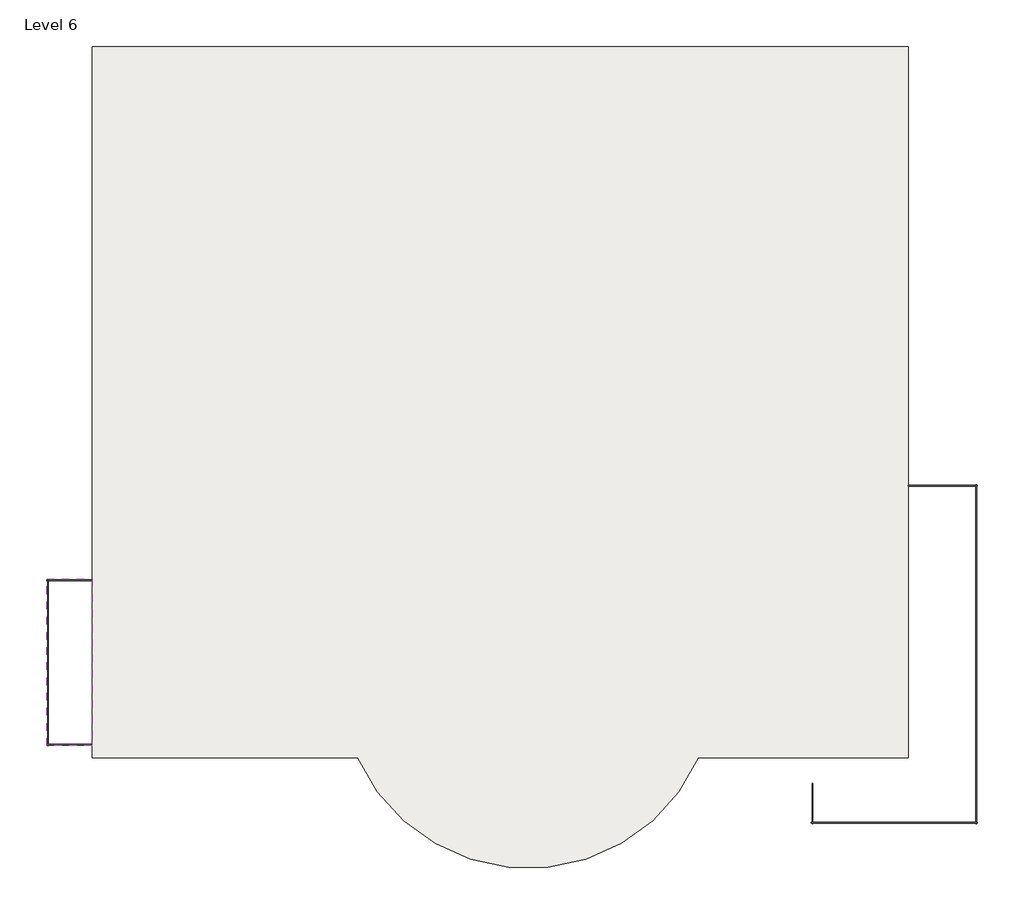
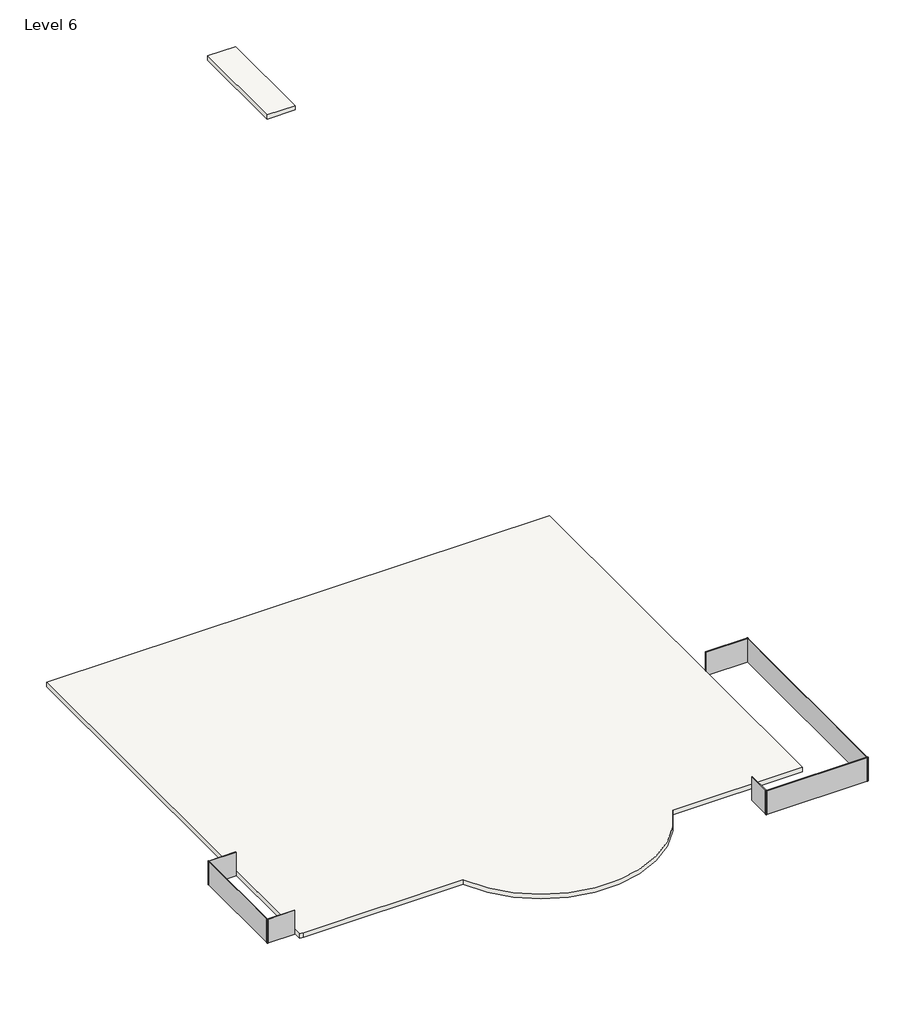
# One storey: 7 plates, 2 slabs.
"""IFC4 building model written with IfcOpenShell, lengths in millimetres."""

from ifc_helpers import new_model, si_unit, point, frame, frame_2d, origin, place, context, project, spatial, polyline, circle_curve, trimmed, segment, composite_curve, outline, extrude, transform, mapped, element, save
from components import system_panel_glazed_7d767388, system_panel_glazed_21a5631f, system_panel_glazed_a5f349e9, system_panel_glazed_84cf4e26, system_panel_glazed_524a14c5, system_panel_glazed_4fcd3a06

model = new_model("IFC4")

# Units and contexts
model_context = context("Model", 3, world=origin())
ifc_project = project(units=[si_unit("LENGTHUNIT", "METRE", prefix="MILLI")], contexts=[model_context])

# Site, building, storey
site = spatial("IfcSite", under=ifc_project)
building = spatial("IfcBuilding", under=site)
storey = spatial("IfcBuildingStorey", under=building, Name="Level 6", Elevation=9601.2)

# Plates
placement = place(None, origin())
system_panel_glazed_shape = system_panel_glazed_7d767388(model_context)
element("IfcPlate", 1, ObjectType="System Panel : Glazed", at=placement, inside=storey, context=model_context, shape_type="MappedRepresentation", body=[
    mapped(system_panel_glazed_shape, transform((-17306.4505427, -8690.0239591, 9601.2), x_axis=(-1.0, 0.0, 0.0), y_axis=(0.0, -1.0, 0.0), z_axis=(0.0, 0.0, 1.0))),
])
element("IfcPlate", 2, ObjectType="System Panel : Glazed", at=placement, inside=storey, context=model_context, shape_type="MappedRepresentation", body=[
    mapped(system_panel_glazed_shape, transform((-17306.4505427, -13712.8739591, 9601.2), x_axis=(1.0, 0.0, 0.0), y_axis=(0.0, 1.0, 0.0), z_axis=(0.0, 0.0, 1.0))),
])
system_panel_glazed_2_shape = system_panel_glazed_21a5631f(model_context)
element("IfcPlate", 3, ObjectType="System Panel : Glazed", at=placement, inside=storey, context=model_context, shape_type="MappedRepresentation", body=[
    mapped(system_panel_glazed_2_shape, transform((7560.1494573, -16059.2808221, 9601.2), x_axis=(1.0, 0.0, 0.0), y_axis=(0.0, 1.0, 0.0), z_axis=(0.0, 0.0, 1.0))),
])
system_panel_glazed_3_shape = system_panel_glazed_a5f349e9(model_context)
element("IfcPlate", 4, ObjectType="System Panel : Glazed", at=placement, inside=storey, context=model_context, shape_type="MappedRepresentation", body=[
    mapped(system_panel_glazed_3_shape, transform((-17979.5505427, -11201.4489591, 9601.2), x_axis=(0.0, -1.0, 0.0), y_axis=(1.0, 0.0, 0.0), z_axis=(0.0, 0.0, 1.0))),
])
system_panel_glazed_4_shape = system_panel_glazed_84cf4e26(model_context)
element("IfcPlate", 5, ObjectType="System Panel : Glazed", at=placement, inside=storey, context=model_context, shape_type="MappedRepresentation", body=[
    mapped(system_panel_glazed_4_shape, transform((5058.2494573, -15449.6808221, 9601.2), x_axis=(0.0, -1.0, 0.0), y_axis=(1.0, 0.0, 0.0), z_axis=(0.0, 0.0, 1.0))),
])
system_panel_glazed_5_shape = system_panel_glazed_524a14c5(model_context)
element("IfcPlate", 6, ObjectType="System Panel : Glazed", at=placement, inside=storey, context=model_context, shape_type="MappedRepresentation", body=[
    mapped(system_panel_glazed_5_shape, transform((10062.0494573, -10953.8808221, 9601.2), x_axis=(0.0, 1.0, 0.0), y_axis=(-1.0, 0.0, 0.0), z_axis=(0.0, 0.0, 1.0))),
])
system_panel_glazed_6_shape = system_panel_glazed_4fcd3a06(model_context)
element("IfcPlate", 7, ObjectType="System Panel : Glazed", at=placement, inside=storey, context=model_context, shape_type="MappedRepresentation", body=[
    mapped(system_panel_glazed_6_shape, transform((9020.6494573, -5848.4808221, 9601.2), x_axis=(-1.0, 0.0, 0.0), y_axis=(0.0, -1.0, 0.0), z_axis=(0.0, 0.0, 1.0))),
])

# Slabs
element("IfcSlab", 8, ObjectType="9\"", at=placement, inside=storey, context=model_context, shape_type="SweptSolid", body=[
    extrude(outline(composite_curve([segment(polyline([(-16607.9505427, 7359.5191779), (7979.2494573, 7359.5191779), (7979.2494573, -14078.0808221), (1652.8739931, -14078.0808221)]), True, "CONTINUOUS"), segment(trimmed(circle_curve(frame_2d((-3476.1505427, -11788.3650223)), 5616.9111737), [point((1652.8739931, -14078.0808221))], [point((-8605.1750786, -14078.0808221))], False, "CARTESIAN"), True, "CONTINUOUS"), segment(polyline([(-8605.1750786, -14078.0808221), (-16404.7505427, -14078.0808221), (-16607.9505427, -14078.0808221), (-16607.9505427, 7359.5191779)]), True, "CONTINUOUS")], self_intersect=False)), frame((0.0, 0.0, 9601.2), z_axis=(0.0, 0.0, 1.0), x_axis=(1.0, 0.0, 0.0)), (0.0, 0.0, 1.0), 228.6),
])
element("IfcSlab", 9, ObjectType="9\"", at=placement, inside=storey, context=model_context, shape_type="SweptSolid", body=[
    extrude(outline(polyline([(-17989.9345352, -8690.0239591), (-16618.3345352, -8690.0239591), (-16618.3345352, -13719.2239591), (-17989.9345352, -13719.2239591), (-17989.9345352, -8690.0239591)])), frame((0.0, 0.0, 52197.0), z_axis=(0.0, 0.0, 1.0), x_axis=(1.0, 0.0, 0.0)), (0.0, 0.0, 1.0), 228.6),
])

save(model, "model.ifc")

# Revit data of these elements
# Type "System Panel : Glazed"
#   Construction Type Id = "GSP4R"
#   Analytic Construction = "1/8 in Pilkington single glazing"
#   Visual Light Transmittance = 0.9
#   Solar Heat Gain Coefficient = 0.86
#   Heat Transfer Coefficient (U) = 1.18115 BTU/(h·ft²·°F)
# Type "9\""
#   Assembly Code = "B1010"
#   Function = 0
#   Layers, outside or top first: 0' - 9" no material (function 1)
# Elements 1, 2, 3, 4, 5, 6, 7 (IfcPlate, "System Panel : Glazed")
#   Phase Created = New Construction
#   Materials on its faces: "Glass"
# Element 8 (IfcSlab, "9\"")
#   built-in parameter 1001955 = 1.5708 (stored number, unit not read)
#   Height Offset From Level = 0' - 9"
#   Phase Created = New Construction
#   Materials on its faces: "Default Floor"
# Element 9 (IfcSlab, "9\"")
#   built-in parameter 1001955 = 3.14159 (stored number, unit not read)
#   Height Offset From Level = 140' - 6"
#   Phase Created = New Construction
#   Materials on its faces: "Default Floor"
# Materials
#   "Glass": class "Glass", colour RGB 0 128 192, transparency 0.75, Description = "Soda Lime Glass", Cost = 0
#   "Default Floor": colour RGB 128 128 128, transparency 0
